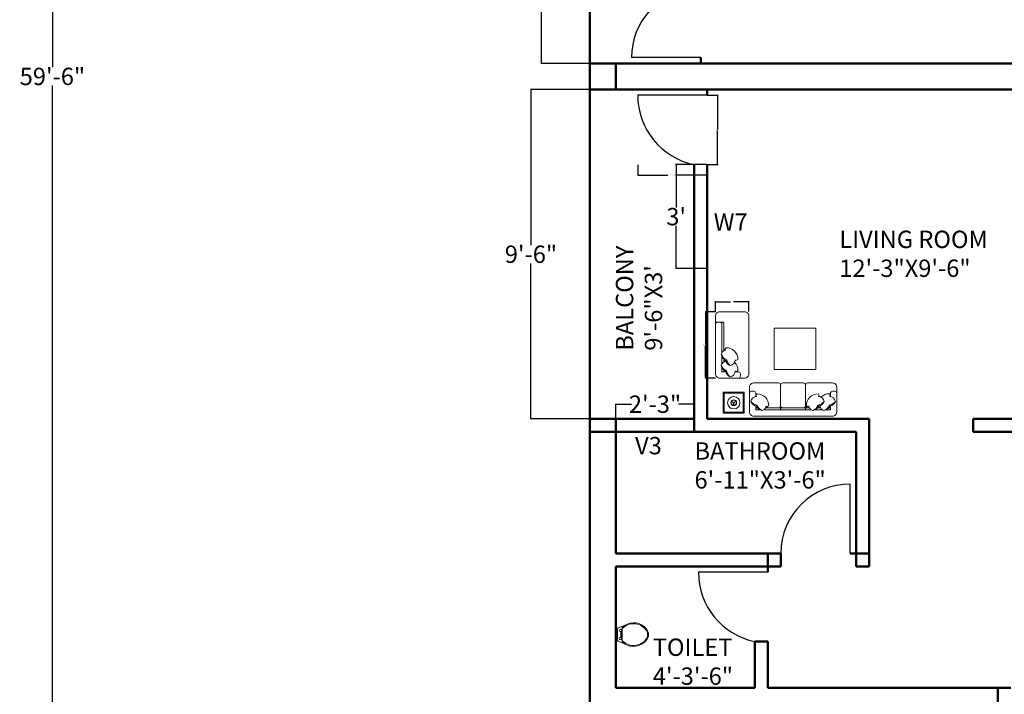
# Model space of a CAD drawing. Units: inches. Extents: x -173 to 545, y -746 to 104.
# Tile 2 of 32: x -173 to 168, y -554 to -321. Entities that reach past the tile are written whole.
import ezdxf

# ---------------------------------------------------------------- set-up
doc = ezdxf.new("R2010")
doc.units = ezdxf.units.IN
doc.header["$MEASUREMENT"] = 0
for name, color, linetype, lineweight in [('A-ANNO-DIMS', 2, 'Continuous', 18), ('A-ANNO-TEXT', 7, 'Continuous', 18), ('A-AREA-IDEN', 7, 'Continuous', 18), ('A-DOOR', 4, 'Continuous', 25), ('A-FLOR-FIXT', 8, 'Continuous', 18), ('A-FURN', 8, 'Continuous', 18), ('A-GLAZ', 3, 'Continuous', 25), ('A-WALL', 7, 'Continuous', 50)]:
    doc.layers.add(name, color=color, linetype=linetype, lineweight=lineweight)
doc.styles.get("Standard").update_dxf_attribs({"font": 'arial.ttf'})
doc.dimstyles.get("Standard").update_dxf_attribs({"dimtxt": 0.18, "dimasz": 0.18, "dimexe": 0.18, "dimexo": 0.0625, "dimgap": 0.09, "dimtad": 0, "dimtih": 1, "dimtoh": 1, "dimdec": 0, "dimzin": 0, "dimdsep": 46, "dimlunit": 3, "dimtxsty": 'Standard', "dimcen": 0.09, "dimadec": 0, "dimazin": 0, "dimtfac": 1, "dimtdec": 0, "dimtofl": 0, "dimtmove": 0, "dimatfit": 3, "dimfxl": 1, "dimtolj": 1, "dimtzin": 0, "dimarcsym": 0})

# ---------------------------------------------------------------- blocks, each defined once
blk = doc.blocks.new('*D7')
at = {"layer": 'A-ANNO-DIMS', "color": 0, "lineweight": -2, "transparency": 16777216}
for p, q in [((24.24, -221.86), (7.32, -221.86)), ((7.5, -222.04), (7.5, -275.71)), ((7.5, -335.68), (7.5, -282.02)), ((24.24, -335.86), (7.32, -335.86))]:
    blk.add_line(p, q, dxfattribs=at)
at = {"layer": 'A-ANNO-DIMS', "color": 0, "transparency": 16777216}
for points in [[(7.47, -222.04), (7.53, -222.04), (7.5, -221.86)], [(7.47, -335.68), (7.53, -335.68), (7.5, -335.86)]]:
    blk.add_solid(points, dxfattribs=at)
at = {"layer": 'Defpoints', "color": 0, "transparency": 16777216}
for p in [(24.3, -221.86), (7.5, -335.86), (24.3, -335.86)]:
    blk.add_point(p, dxfattribs=at)
at = {"layer": 'A-ANNO-DIMS', "color": 0, "transparency": 16777216, "insert": (7.5, -278.86), "char_height": 6, "attachment_point": 5}
blk.add_mtext('\\A1;9\'-6"', dxfattribs=at)
blk = doc.blocks.new('*D11')
at = {"layer": 'A-ANNO-DIMS', "color": 0, "lineweight": -2, "transparency": 16777216}
for p, q in [((60.24, -370.86), (53.92, -370.86)), ((54.1, -371.04), (54.1, -385.71)), ((54.1, -406.68), (54.1, -392.02)), ((60.24, -406.86), (53.92, -406.86))]:
    blk.add_line(p, q, dxfattribs=at)
at = {"layer": 'A-ANNO-DIMS', "color": 0, "transparency": 16777216}
for points in [[(54.07, -371.04), (54.13, -371.04), (54.1, -370.86)], [(54.07, -406.68), (54.13, -406.68), (54.1, -406.86)]]:
    blk.add_solid(points, dxfattribs=at)
at = {"layer": 'Defpoints', "color": 0, "transparency": 16777216}
for p in [(60.3, -370.86), (54.1, -406.86), (60.3, -406.86)]:
    blk.add_point(p, dxfattribs=at)
at = {"layer": 'A-ANNO-DIMS', "color": 0, "transparency": 16777216, "insert": (54.1, -388.86), "char_height": 6, "attachment_point": 5}
blk.add_mtext("\\A1;3'", dxfattribs=at)
blk = doc.blocks.new('*D12')
at = {"layer": 'A-ANNO-DIMS', "color": 0, "lineweight": -2, "transparency": 16777216}
for p, q in [((24.24, -344.86), (3.72, -344.86)), ((3.9, -345.04), (3.9, -398.71)), ((3.9, -458.68), (3.9, -405.02)), ((24.24, -458.86), (3.72, -458.86))]:
    blk.add_line(p, q, dxfattribs=at)
at = {"layer": 'A-ANNO-DIMS', "color": 0, "transparency": 16777216}
for points in [[(3.87, -345.04), (3.93, -345.04), (3.9, -344.86)], [(3.87, -458.68), (3.93, -458.68), (3.9, -458.86)]]:
    blk.add_solid(points, dxfattribs=at)
at = {"layer": 'Defpoints', "color": 0, "transparency": 16777216}
for p in [(24.3, -344.86), (3.9, -458.86), (24.3, -458.86)]:
    blk.add_point(p, dxfattribs=at)
at = {"layer": 'A-ANNO-DIMS', "color": 0, "transparency": 16777216, "insert": (3.9, -401.86), "char_height": 6, "attachment_point": 5}
blk.add_mtext('\\A1;9\'-6"', dxfattribs=at)
blk = doc.blocks.new('*D14')
at = {"layer": 'A-ANNO-DIMS', "color": 0, "lineweight": -2, "transparency": 16777216}
for p, q in [((33.3, -458.8), (33.3, -453.57)), ((33.48, -453.75), (38.69, -453.75)), ((60.12, -453.75), (54.92, -453.75)), ((60.3, -458.8), (60.3, -453.57))]:
    blk.add_line(p, q, dxfattribs=at)
at = {"layer": 'A-ANNO-DIMS', "color": 0, "transparency": 16777216}
for points in [[(33.48, -453.72), (33.48, -453.78), (33.3, -453.75)], [(60.12, -453.72), (60.12, -453.78), (60.3, -453.75)]]:
    blk.add_solid(points, dxfattribs=at)
at = {"layer": 'Defpoints', "color": 0, "transparency": 16777216}
for p in [(60.3, -453.75), (33.3, -458.86), (60.3, -458.86)]:
    blk.add_point(p, dxfattribs=at)
at = {"layer": 'A-ANNO-DIMS', "color": 0, "transparency": 16777216, "insert": (46.8, -453.75), "char_height": 6, "attachment_point": 5}
blk.add_mtext('\\A1;2\'-3"', dxfattribs=at)
blk = doc.blocks.new('DAY BED1')
at = {"color": 0}
blk.add_line((0.3, 0.25), (0.225, 0.255), dxfattribs=at)
blk.add_lwpolyline([(-0.3, 0, -0.414214), (-0.4, 0.1), (-0.4, 0.1, 0.317837), (-0.4, 0.1, -0.414214), (-0.4, 0.1), (-0.4, 0.1, 1.186185), (-0.4, 0.1, -0.414214), (-0.4, 0.1), (-0.4, 1.5, -0.414214), (-0.3, 1.6), (0.3, 1.6, -0.414214), (0.4, 1.5), (0.4, 0.1, -0.414214), (0.3, 0)], format="xyb", close=True, dxfattribs=at)
for points in [[(-0.073, 1.45), (-0.15, 1.45, -0.414214), (-0.2, 1.5), (-0.2, 1.55, -0.414214), (-0.15, 1.6)], [(-0.073, 1.45, 0.165541), (-0.139, 1.419, 0.200231), (-0.058, 1.221, 0.121523)], [(-0.076, 1.425, -0.356772), (0.05, 1.568, -0.249542), (0.154, 1.438, 9.61688)], [(0.05, 1.568, -0.14773), (0.136, 1.422, -0.213343), (0.262, 1.293, -0.178662)], [(0.143, 1.442, -0.306663), (0.262, 1.293, -0.30633), (0.154, 1.196, 0.872847)], [(0.25, 1.345), (0.25, 1.45), (0.152, 1.45, -0.414214)], [(0.2, 1.412), (0.2, 1.43, -0.414214), (0.22, 1.45), (0.23, 1.45, -0.414214), (0.25, 1.43)], [(0.25, 1.43), (0.25, 1.345, -0.414214)], [(-0.076, 1.156, -0.356772), (0.05, 1.299, -0.249542), (0.154, 1.169, 9.61688)], [(0.05, 1.299, -0.14773), (0.136, 1.153, -0.213343), (0.262, 1.024, -0.178662)], [(0.168, 1.163, 0.071865), (0.187, 1.205, -7.115464)], [(0.2, 1.142), (0.2, 1.211, -0.414214)], [(0.25, 1.262), (0.25, 1.075, -0.414214)], [(-0.073, 1.181, 0.165541), (-0.139, 1.15, 0.425989), (0.148, 0.869, 0.121523), (0.187, 0.936, -7.115464)], [(0.143, 1.173, -0.306663), (0.262, 1.024, -0.30633), (0.154, 0.926, 0.872847)], [(0.25, 0.992), (0.25, 0.275, -0.414214), (0.23, 0.255), (0.22, 0.255, -0.414214), (0.2, 0.275), (0.2, 0.942, -0.414214)], [(0.25, 0.377), (0.25, 0.3, 0.414214), (0.3, 0.25), (0.35, 0.25, 0.414214), (0.4, 0.3)]]:
    blk.add_lwpolyline(points, format="xyb", dxfattribs=at)
for points in [[(0.25, 1.075), (0.25, 1.262)], [(0.25, 0.377), (0.25, 0.992)]]:
    blk.add_lwpolyline(points, dxfattribs=at)
blk = doc.blocks.new('*D24')
at = {"layer": 'A-ANNO-DIMS', "color": 0, "lineweight": -2, "transparency": 16777216}
for p, q in [((24.24, 16.64), (-161.72, 16.64)), ((-161.54, 16.46), (-161.54, -337.21)), ((-161.54, -697.18), (-161.54, -343.52)), ((24.24, -697.36), (-161.72, -697.36))]:
    blk.add_line(p, q, dxfattribs=at)
at = {"layer": 'A-ANNO-DIMS', "color": 0, "transparency": 16777216}
for points in [[(-161.57, 16.46), (-161.51, 16.46), (-161.54, 16.64)], [(-161.57, -697.18), (-161.51, -697.18), (-161.54, -697.36)]]:
    blk.add_solid(points, dxfattribs=at)
at = {"layer": 'Defpoints', "color": 0, "transparency": 16777216}
for p in [(24.3, 16.64), (-161.54, -697.36), (24.3, -697.36)]:
    blk.add_point(p, dxfattribs=at)
at = {"layer": 'A-ANNO-DIMS', "color": 0, "transparency": 16777216, "insert": (-161.54, -340.36), "char_height": 6, "attachment_point": 5}
blk.add_mtext('\\A1;59\'-6"', dxfattribs=at)
blk = doc.blocks.new('WC-COMPACT')
for p, q in [((1.62, 6.19), (1.62, 6.64)), ((1.62, 6.19), (1.62, 4.09)), ((1.62, 1.98), (1.62, 4.09)), ((1.62, 1.53), (1.62, 1.98))]:
    blk.add_line(p, q)
for points in [[(0, 4.09), (0, 6.13, -0.31031), (0.17, 6.38), (2.36, 7.22, -0.209071)], [(1.62, 6.19, -0.448546), (9.69, 5.9, -0.162618), (10.38, 4.09, -0.470877)], [(1.62, 6.64, -0.040937), (2.36, 7.22, -0.163732)], [(2.36, 7.22, -0.383919), (9.93, 6.1, -0.163732), (10.7, 4.09, -0.359733)], [(0, 4.09), (0, 2.04, 0.31031), (0.17, 1.79), (2.36, 0.95, 0.209071)], [(1.3, 5.82), (0.85, 5.82, 1), (0.85, 5.14), (1.08, 5.14)], [(1.3, 5.82, -0.022712), (1.62, 6.19, -0.162618)], [(1.3, 4.09), (1.3, 5.82, -0.476108)], [(1.3, 4.09), (1.3, 2.35, 0.022712)], [(1.84, 1.77, 0.431639), (9.69, 2.28, 0.162618), (10.38, 4.09, 0.470877)], [(2.36, 0.95, 0.383919), (9.93, 2.08, 0.163732), (10.7, 4.09, 0.359733)], [(1.3, 2.35), (0.85, 2.35, -1), (0.85, 3.03), (1.08, 3.03)], [(1.3, 2.35, 0.022712), (1.62, 1.98, 0.162618)], [(1.62, 1.98, 0.014165), (1.84, 1.77, 0.162618)], [(1.62, 1.53, 0.040937), (2.36, 0.95, 0.163732)]]:
    blk.add_lwpolyline(points, format="xyb")
for points in [[(1.08, 5.14), (1.08, 3.03)], [(1.08, 5.14), (1.3, 5.14)], [(1.08, 3.03), (1.3, 3.03)]]:
    blk.add_lwpolyline(points)
blk = doc.blocks.new('DOOR-24')
blk.add_line((24, 0), (24, 24))
blk.add_arc((24, 0), 24, 90, 180)
blk = doc.blocks.new('DOOR-24-OFFSET')
blk.add_line((24, 24), (0, 24))
blk.add_arc((24.52, 24), 24.52, 180, 258.1877)
blk = doc.blocks.new('*D48')
at = {"layer": 'A-ANNO-DIMS', "color": 0, "lineweight": -2, "transparency": 16777216}
for p, q in [((67.65, -421.76), (64.09, -421.76)), ((64.27, -421.94), (64.27, -433.06)), ((64.27, -444.54), (64.27, -433.42)), ((67.65, -444.72), (64.09, -444.72))]:
    blk.add_line(p, q, dxfattribs=at)
at = {"layer": 'A-ANNO-DIMS', "color": 0, "transparency": 16777216}
for points in [[(64.24, -421.94), (64.3, -421.94), (64.27, -421.76)], [(64.24, -444.54), (64.3, -444.54), (64.27, -444.72)]]:
    blk.add_solid(points, dxfattribs=at)
at = {"layer": 'Defpoints', "color": 0, "transparency": 16777216}
for p in [(67.72, -421.76), (64.27, -444.72), (67.72, -444.72)]:
    blk.add_point(p, dxfattribs=at)
at = {"layer": 'A-ANNO-DIMS', "color": 0, "transparency": 16777216, "insert": (64.27, -433.24), "char_height": 0.18, "attachment_point": 5}
blk.add_mtext('\\A1;DAY BED 1\'-11"', dxfattribs=at)
blk = doc.blocks.new('*D49')
at = {"layer": 'A-ANNO-DIMS', "color": 0, "lineweight": -2, "transparency": 16777216}
for p, q in [((67.72, -421.69), (67.72, -418.13)), ((67.9, -418.31), (72.85, -418.31)), ((79.02, -418.31), (74.06, -418.31)), ((79.2, -421.69), (79.2, -418.13))]:
    blk.add_line(p, q, dxfattribs=at)
at = {"layer": 'A-ANNO-DIMS', "color": 0, "transparency": 16777216}
for points in [[(67.9, -418.28), (67.9, -418.34), (67.72, -418.31)], [(79.02, -418.28), (79.02, -418.34), (79.2, -418.31)]]:
    blk.add_solid(points, dxfattribs=at)
at = {"layer": 'Defpoints', "color": 0, "transparency": 16777216}
for p in [(67.72, -418.31), (67.72, -421.76), (79.2, -421.76)]:
    blk.add_point(p, dxfattribs=at)
at = {"layer": 'A-ANNO-DIMS', "color": 0, "transparency": 16777216, "insert": (73.46, -418.31), "char_height": 0.18, "attachment_point": 5}
blk.add_mtext('\\A1;0\'-11 1/2"', dxfattribs=at)
blk = doc.blocks.new('*D58')
at = {"layer": 'A-ANNO-DIMS', "color": 0, "lineweight": -2, "transparency": 16777216}
for p, q in [((40.8, -370.92), (40.8, -374.64)), ((64.8, -370.92), (64.8, -374.64)), ((40.98, -374.46), (51.22, -374.46)), ((64.62, -374.46), (54.38, -374.46))]:
    blk.add_line(p, q, dxfattribs=at)
at = {"layer": 'A-ANNO-DIMS', "color": 0, "transparency": 16777216}
for points in [[(40.98, -374.43), (40.98, -374.49), (40.8, -374.46)], [(64.62, -374.43), (64.62, -374.49), (64.8, -374.46)]]:
    blk.add_solid(points, dxfattribs=at)
at = {"layer": 'Defpoints', "color": 0, "transparency": 16777216}
for p in [(40.8, -370.86), (64.8, -370.86), (64.8, -374.46)]:
    blk.add_point(p, dxfattribs=at)
at = {"layer": 'A-ANNO-DIMS', "color": 0, "transparency": 16777216, "insert": (52.8, -374.46), "char_height": 0.18, "attachment_point": 5}
blk.add_mtext('\\A1;OFFSET DOOR 2\'-0" TYP.', dxfattribs=at)
blk = doc.blocks.new('*D59')
at = {"layer": 'A-ANNO-DIMS', "color": 0, "lineweight": -2, "transparency": 16777216}
for p, q in [((64.86, -346.86), (68.58, -346.86)), ((68.4, -347.04), (68.4, -358.68)), ((68.4, -370.68), (68.4, -359.04)), ((64.86, -370.86), (68.58, -370.86))]:
    blk.add_line(p, q, dxfattribs=at)
at = {"layer": 'A-ANNO-DIMS', "color": 0, "transparency": 16777216}
for points in [[(68.37, -347.04), (68.43, -347.04), (68.4, -346.86)], [(68.37, -370.68), (68.43, -370.68), (68.4, -370.86)]]:
    blk.add_solid(points, dxfattribs=at)
at = {"layer": 'Defpoints', "color": 0, "transparency": 16777216}
for p in [(64.8, -346.86), (68.4, -346.86), (64.8, -370.86)]:
    blk.add_point(p, dxfattribs=at)
at = {"layer": 'A-ANNO-DIMS', "color": 0, "transparency": 16777216, "insert": (68.4, -358.86), "char_height": 0.18, "attachment_point": 5}
blk.add_mtext('\\A1;2\'-0" TYP.', dxfattribs=at)

msp = doc.modelspace()

# ---------------------------------------------------------------- linework, layer by layer
at = {"layer": 'A-DOOR'}
msp.add_line((62.64, -333.86), (38.64, -333.86), dxfattribs=at)
msp.add_arc((62.77, -333.86), 24.13, 95.876, 180, dxfattribs=at)
at = {"layer": 'A-FURN'}
for p, q in [((74.02, -453.19), (73.14, -452.69)), ((73.97, -453.19), (74.85, -452.69)), ((73.97, -453.27), (73.1, -452.77)), ((73.95, -453.23), (73.95, -454.24)), ((74.02, -453.27), (74.89, -452.77)), ((74.04, -453.23), (74.04, -454.24))]:
    msp.add_line(p, q, dxfattribs=at)
at = {"layer": 'A-FURN', "ltscale": 0.03}
for points in [[(102.34, -427.4), (87.99, -427.4), (87.99, -441.75), (102.34, -441.75)], [(70.41, -449.64), (77.58, -449.64), (77.58, -456.82), (70.41, -456.82)]]:
    msp.add_lwpolyline(points, close=True, dxfattribs=at)
msp.add_lwpolyline([(79.47, -447.83, -0.414214), (80.9, -446.4), (89.51, -446.4, -0.414214), (90.23, -447.11, -0.414214), (90.95, -446.4), (98.12, -446.4, -0.414214), (98.84, -447.11, -0.414214), (99.56, -446.4), (108.17, -446.4, -0.414214), (109.61, -447.83), (109.61, -456.44, -0.414214), (108.17, -457.88), (80.9, -457.88, -0.414214), (79.47, -456.44)], format="xyb", close=True, dxfattribs=at)
at = {"layer": 'A-FURN'}
for points in [[(79.47, -449.98, -0.414214), (80.19, -449.27), (80.9, -449.27, -0.414214), (81.62, -449.98), (81.62, -451.09)], [(89.51, -455.01, 0.414214), (90.23, -454.29), (90.23, -447.11, 0.414214)], [(99.56, -455.01, -0.414214), (98.84, -454.29), (98.84, -447.11, -0.414214)], [(107.45, -451.09), (107.45, -449.98, -0.414214), (108.17, -449.27), (108.89, -449.27, -0.414214), (109.61, -449.98)], [(81.98, -451.05, 0.356772), (79.92, -452.86, 0.249542), (81.79, -454.35, -9.61688)], [(81.62, -451.1, -0.165541), (82.06, -450.15, -0.425989), (86.09, -454.26, -0.121523), (85.14, -454.82, 7.115464)], [(103.59, -451.1, 0.165541), (103.15, -450.15, 0.425989), (99.12, -454.26, 0.121523), (100.07, -454.82, -7.115464)], [(103.23, -451.05, -0.356772), (105.28, -452.86, -0.249542), (103.42, -454.35, 9.61688)], [(107.45, -451.1, 0.165541), (107.01, -450.15, 0.200231), (104.16, -451.3, 0.121523)], [(107.09, -451.05, -0.356772), (109.15, -452.86, -0.249542), (107.29, -454.35, 9.61688)], [(79.92, -452.86, 0.14773), (82.02, -454.09, 0.213343), (83.87, -455.9, 0.178662)], [(82.17, -455.01), (81.91, -455.01, 0.414214), (81.62, -455.29), (81.62, -455.44, 0.414214), (81.91, -455.72)], [(81.73, -454.19, 0.306663), (83.87, -455.9, 0.30633), (85.27, -454.34, -0.872847)], [(81.91, -455.72), (83.13, -455.72, 0.414214)], [(84.32, -455.72), (89.94, -455.72, 0.414214), (90.23, -455.44), (90.23, -455.29, 0.414214), (89.94, -455.01), (85.05, -455.01, 0.414214)], [(90.95, -455.01, -0.414214), (90.23, -454.29)], [(98.12, -455.01, 0.414214), (98.84, -454.29)], [(100.88, -455.72), (99.13, -455.72, -0.414214), (98.84, -455.44), (98.84, -455.29, -0.414214), (99.13, -455.01), (100.16, -455.01, -0.414214)], [(103.48, -454.19, -0.306663), (101.34, -455.9, -0.30633), (99.94, -454.34, 0.872847)], [(105.28, -452.86, -0.14773), (103.19, -454.09, -0.213343), (101.34, -455.9, -0.178662)], [(104.75, -455.72), (102.08, -455.72, -0.414214)], [(103.04, -455.01), (104.03, -455.01, -0.414214)], [(103.34, -454.54, 0.071865), (103.94, -454.82, -7.115464)], [(107.34, -454.19, -0.306663), (105.2, -455.9, -0.30633), (103.8, -454.34, 0.872847)], [(109.15, -452.86, -0.14773), (107.05, -454.09, -0.213343), (105.2, -455.9, -0.178662)], [(105.94, -455.72), (107.45, -455.72), (107.45, -454.31, -0.414214)], [(107.17, -455.72), (105.94, -455.72, -0.414214)], [(106.91, -455.01), (107.17, -455.01, -0.414214), (107.45, -455.29), (107.45, -455.44, -0.414214), (107.17, -455.72)]]:
    msp.add_lwpolyline(points, format="xyb", dxfattribs=at)
msp.add_lwpolyline([(77.3, -449.93), (70.69, -449.93), (70.69, -456.53), (77.3, -456.53)], close=True, dxfattribs=at)
for points in [[(81.62, -454.31), (81.62, -455.72), (83.13, -455.72)], [(84.32, -455.72), (100.88, -455.72)], [(102.08, -455.72), (104.75, -455.72)]]:
    msp.add_lwpolyline(points, dxfattribs=at)
msp.add_lwpolyline([(98.56, -455.72), (90.52, -455.72, -0.414214), (90.23, -455.44), (90.23, -455.29, -0.414214), (90.52, -455.01), (98.56, -455.01, -0.414214), (98.84, -455.29), (98.84, -455.44, -0.414214)], format="xyb", close=True, dxfattribs=at)
for radius in [2.12, 1.01, 0.908]:
    msp.add_circle((74, -453.23), radius, dxfattribs=at)
at = {"layer": 'A-GLAZ'}
for p, q in [((64.8, -370.86), (60.3, -370.86)), ((64.8, -406.86), (60.3, -406.86))]:
    msp.add_line(p, q, dxfattribs=at)
at = {"layer": 'A-WALL'}
for p, q in [((24.3, 16.64), (24.3, -697.36)), ((24.3, -335.86), (219.8, -335.86)), ((33.3, -335.86), (33.3, -344.86)), ((62.64, -335.86), (62.64, -333.86)), ((24.3, -344.86), (219.8, -344.86)), ((64.8, -344.86), (64.8, -346.86)), ((64.8, -344.86), (64.8, -346.86)), ((60.3, -370.86), (60.3, -463.36)), ((64.8, -370.86), (64.8, -458.86)), ((24.3, -458.86), (60.3, -458.86)), ((33.3, -458.86), (33.3, -505.36)), ((64.8, -458.86), (120.8, -458.86)), ((120.8, -458.86), (120.8, -509.86)), ((156.8, -458.86), (156.8, -463.36)), ((156.8, -458.86), (210.8, -458.86)), ((24.3, -463.36), (116.3, -463.36)), ((116.3, -463.36), (116.3, -509.86)), ((156.8, -463.36), (210.8, -463.36)), ((33.3, -505.36), (90.3, -505.36)), ((85.8, -509.86), (85.8, -505.36)), ((90.3, -505.36), (90.3, -509.86)), ((114.3, -505.36), (120.8, -505.36)), ((33.3, -509.86), (90.3, -509.86)), ((33.3, -509.86), (33.3, -551.86)), ((85.8, -509.86), (85.8, -511.86)), ((116.3, -509.86), (120.8, -509.86)), ((81.3, -535.86), (81.3, -551.86)), ((85.8, -535.86), (81.3, -535.86)), ((85.8, -535.86), (85.8, -551.86)), ((33.3, -551.86), (81.3, -551.86)), ((85.8, -551.86), (169.8, -551.86)), ((165.3, -551.86), (165.3, -688.36))]:
    msp.add_line(p, q, dxfattribs=at)

# ---------------------------------------------------------------- block references
at = {"layer": 'A-DOOR'}
for name, p in [('DOOR-24-OFFSET', (40.8, -370.86)), ('DOOR-24', (90.3, -505.36)), ('DOOR-24-OFFSET', (61.8, -535.86))]:
    msp.add_blockref(name, p, dxfattribs=at)
at = {"layer": 'A-FLOR-FIXT'}
msp.add_blockref('WC-COMPACT', (33.86, -537.54), dxfattribs=at)
at = {"layer": 'A-FURN', "ltscale": 0.03, "xscale": 14.35129690169236, "yscale": 14.35129690169236, "zscale": 14.35129690169236, "rotation": 180}
msp.add_blockref('DAY BED1', (73.46, -421.76), dxfattribs=at)

# ---------------------------------------------------------------- texts
at = {"layer": 'A-ANNO-TEXT', "char_height": 6, "attachment_point": 1}
for s, insert in [('W7', (67.08, -387.72)), ('V3', (39.9, -465.09))]:
    msp.add_mtext(s, dxfattribs=dict(at, insert=insert))
at = {"layer": 'A-AREA-IDEN', "char_height": 6, "attachment_point": 1}
for s, insert in [('LIVING ROOM\\P12\'-3"X9\'-6"', (110.5, -393.72)), ('BATHROOM\\P6\'-11"X3\'-6"', (60.44, -466.93)), ('TOILET\\P4\'-3\'-6"', (46.02, -534.82))]:
    msp.add_mtext(s, dxfattribs=dict(at, insert=insert))
at = {"layer": 'A-AREA-IDEN', "insert": (33.27, -435.23), "char_height": 6, "attachment_point": 1, "rotation": 90}
msp.add_mtext('BALCONY\\P9\'-6"X3\'', dxfattribs=at)

# ---------------------------------------------------------------- dimensions: what is measured, and where the dimension line sits
at = {"layer": 'A-ANNO-DIMS'}
for base, p1, p2, angle, override, picture, middle in [((-161.54, -697.36), (24.3, 16.64), (24.3, -697.36), 90, {"dimtxt": 6, "dimclrd": 0, "dimclre": 0, "dimclrt": 0}, '*D24', (-161.54, -340.36)), ((7.5, -335.86), (24.3, -221.86), (24.3, -335.86), 90, {"dimtxt": 6, "dimclrd": 0, "dimclre": 0, "dimclrt": 0}, '*D7', (7.5, -278.86)), ((3.9, -458.86), (24.3, -344.86), (24.3, -458.86), 90, {"dimtxt": 6, "dimclrd": 0, "dimclre": 0, "dimclrt": 0}, '*D12', (3.9, -401.86)), ((54.1, -406.86), (60.3, -370.86), (60.3, -406.86), 90, {"dimtxt": 6, "dimclrd": 0, "dimclre": 0, "dimclrt": 0}, '*D11', (54.1, -388.86)), ((67.72, -418.31), (79.2, -421.76), (67.72, -421.76), 180, {"dimdec": 1, "dimlfac": 1, "dimrnd": 0, "dimzin": 1, "dimdsep": 46, "dimlunit": 4, "dimfrac": 2}, '*D49', (73.46, -418.31))]:
    dim = msp.add_linear_dim(base=base, p1=p1, p2=p2, angle=angle, dimstyle='Standard', override=override, dxfattribs=at)
    dim.commit()
    dim.dimension.update_dxf_attribs({"geometry": picture, "text_midpoint": middle})
for base, p1, p2, angle, text, picture, middle in [((68.4, -346.86), (64.8, -370.86), (64.8, -346.86), 90, '<> TYP.', '*D59', (68.4, -358.86)), ((64.27, -444.72), (67.72, -421.76), (67.72, -444.72), 270, 'DAY BED <>', '*D48', (64.27, -433.24))]:
    dim = msp.add_linear_dim(base=base, p1=p1, p2=p2, angle=angle, text=text, dimstyle='Standard', override={"dimdec": 1, "dimlfac": 1, "dimrnd": 0, "dimzin": 1, "dimdsep": 46, "dimlunit": 4, "dimfrac": 2}, dxfattribs=at)
    dim.commit()
    dim.dimension.update_dxf_attribs({"geometry": picture, "text_midpoint": middle})
dim = msp.add_linear_dim(base=(64.8, -374.46), p1=(40.8, -370.86), p2=(64.8, -370.86), text='OFFSET DOOR <> TYP.', dimstyle='Standard', override={"dimdec": 1, "dimlfac": 1, "dimrnd": 0, "dimzin": 1, "dimdsep": 46, "dimlunit": 4, "dimfrac": 2}, dxfattribs=at)
dim.commit()
dim.dimension.update_dxf_attribs({"geometry": '*D58', "text_midpoint": (52.8, -374.46)})
dim = msp.add_linear_dim(base=(60.3, -453.75), p1=(33.3, -458.86), p2=(60.3, -458.86), dimstyle='Standard', override={"dimtxt": 6, "dimclrd": 0, "dimclre": 0, "dimclrt": 0}, dxfattribs=at)
dim.commit()
dim.dimension.update_dxf_attribs({"geometry": '*D14', "text_midpoint": (46.8, -453.75)})

doc.saveas('drawing.dxf')
